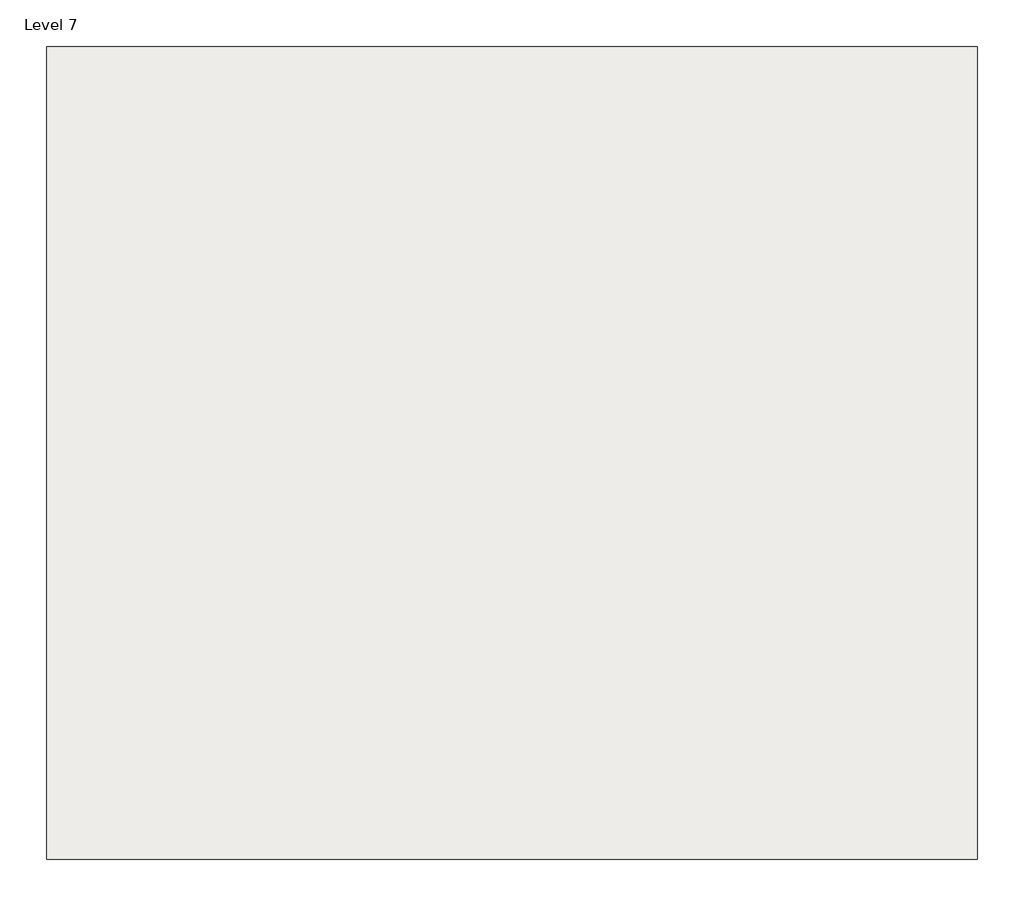
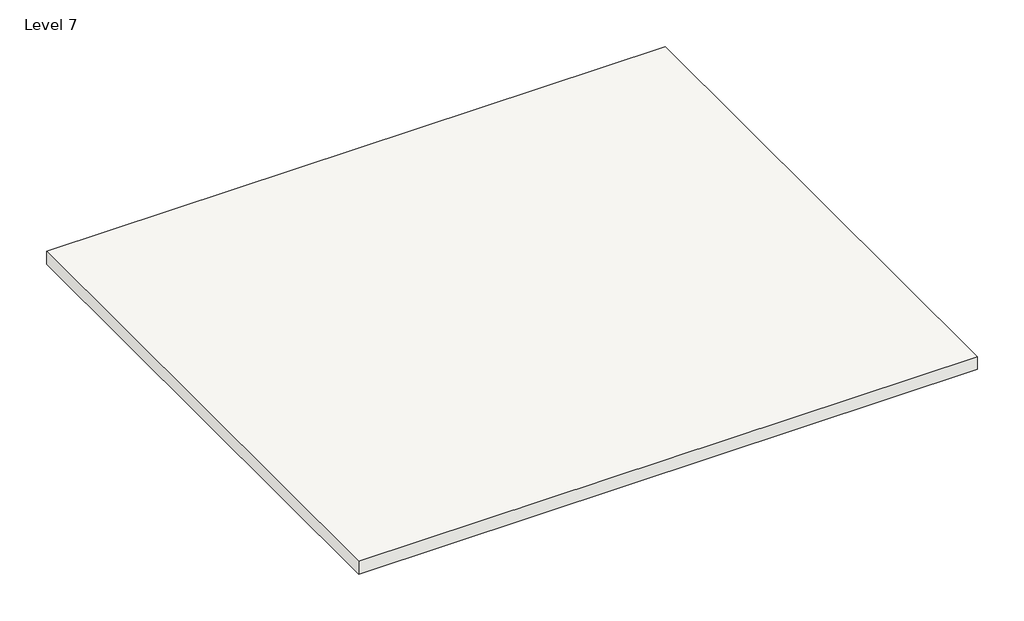
# One storey: 1 slab.
"""IFC4 building model written with IfcOpenShell, lengths in millimetres."""

from ifc_helpers import new_model, si_unit, frame, origin, place, context, project, spatial, polyline, outline, extrude, element, save

model = new_model("IFC4")

# Units and contexts
model_context = context("Model", 3, world=origin())
ifc_project = project(units=[si_unit("LENGTHUNIT", "METRE", prefix="MILLI")], contexts=[model_context])

# Site, building, storey
site = spatial("IfcSite", under=ifc_project)
building = spatial("IfcBuilding", under=site)
storey = spatial("IfcBuildingStorey", under=building, Name="Level 7", Elevation=18288.0)

# Slab
placement = place(None, origin())
element("IfcSlab", 1, ObjectType="Generic - 12\"", at=placement, inside=storey, context=model_context, shape_type="SweptSolid", body=[
    extrude(outline(polyline([(-12404.644627, 6538.6098866), (1819.355373, 6538.6098866), (1819.355373, -5881.9901134), (-12404.644627, -5881.9901134), (-12404.644627, 6538.6098866)])), frame((0.0, 0.0, 18592.8), z_axis=(0.0, 0.0, 1.0), x_axis=(1.0, 0.0, 0.0)), (0.0, 0.0, 1.0), 304.8),
])

save(model, "model.ifc")

# Revit data of these elements
# Type "Generic - 12\""
#   Assembly Code = "B1010"
#   Function = 0
#   Layers, outside or top first: 1' - 0" "Parking Stripe" (function 1)
# Element 1 (IfcSlab, "Generic - 12\"")
#   built-in parameter 1001955 = 3.14159 (stored number, unit not read)
#   Height Offset From Level = 2' - 0"
#   Phase Created = New Construction
#   Materials on its faces: "Parking Stripe"
# Materials
#   "Parking Stripe": class "Paint", colour RGB 250 250 91, transparency 0, Cost = 0
